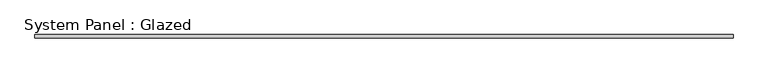
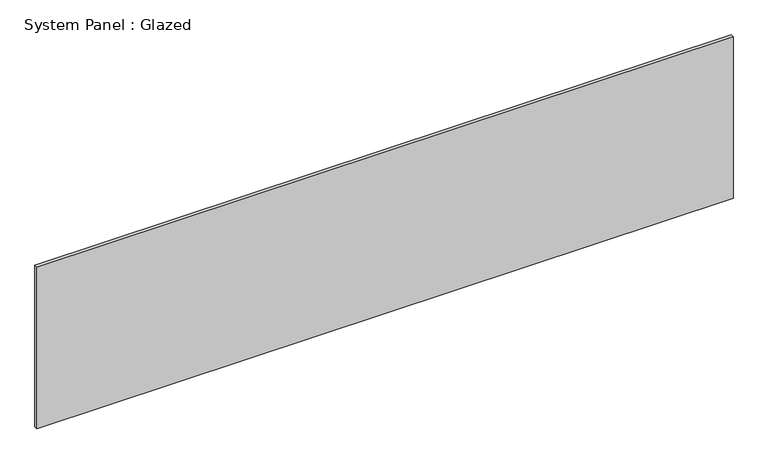
"""IFC4 building model written with IfcOpenShell, lengths in millimetres: plate geometry, System Panel : Glazed."""

from ifc_helpers import new_model, si_unit, origin, origin_with_axes, place, context, project, spatial, polyline, outline, extrude, source, transform, mapped, element, save


def system_panel_glazed_dfd0d0b7(model_context):
    return source(origin(), model_context, "Body", "SweptSolid", [
        extrude(outline(polyline([(2489.2, 19.05), (-2489.2, 19.05), (-2489.2, 44.45), (2489.2, 44.45), (2489.2, 19.05)])), origin_with_axes(), (0.0, 0.0, 1.0), 1219.2),
    ])


if __name__ == "__main__":
    model = new_model("IFC4")
    model_context = context("Model", 3, world=origin())
    ifc_project = project(units=[si_unit("LENGTHUNIT", "METRE", prefix="MILLI")], contexts=[model_context])
    site = spatial("IfcSite", under=ifc_project)
    building = spatial("IfcBuilding", under=site)
    placement = place(None, origin())
    system_panel_glazed_shape = system_panel_glazed_dfd0d0b7(model_context)
    element("IfcPlate", 1, ObjectType="System Panel : Glazed", at=placement, inside=building, context=model_context, shape_type="MappedRepresentation", body=[
        mapped(system_panel_glazed_shape, transform((0.0, 0.0, 0.0), x_axis=(1.0, 0.0, 0.0), y_axis=(0.0, 1.0, 0.0), z_axis=(0.0, 0.0, 1.0))),
    ])
    save(model, "model.ifc")

# Revit data of these elements
# Type "System Panel : Glazed"
#   Construction Type Id = "GSP4R"
#   Analytic Construction = "1/8 in Pilkington single glazing"
#   Visual Light Transmittance = 0.9
#   Solar Heat Gain Coefficient = 0.86
#   Heat Transfer Coefficient (U) = 1.18115 BTU/(h·ft²·°F)
# Element 1 (IfcPlate, "System Panel : Glazed")
#   Materials on its faces: "Glass"
# Materials
#   "Glass": class "Glass", colour RGB 0 128 192, transparency 0.75, Description = "Soda Lime Glass", Cost = 0
